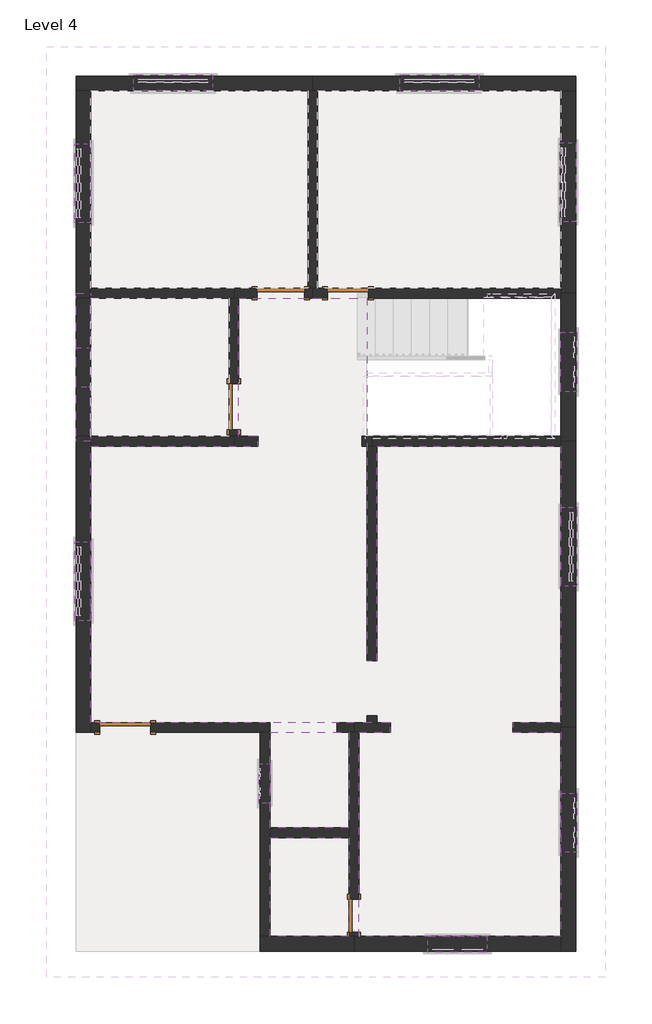
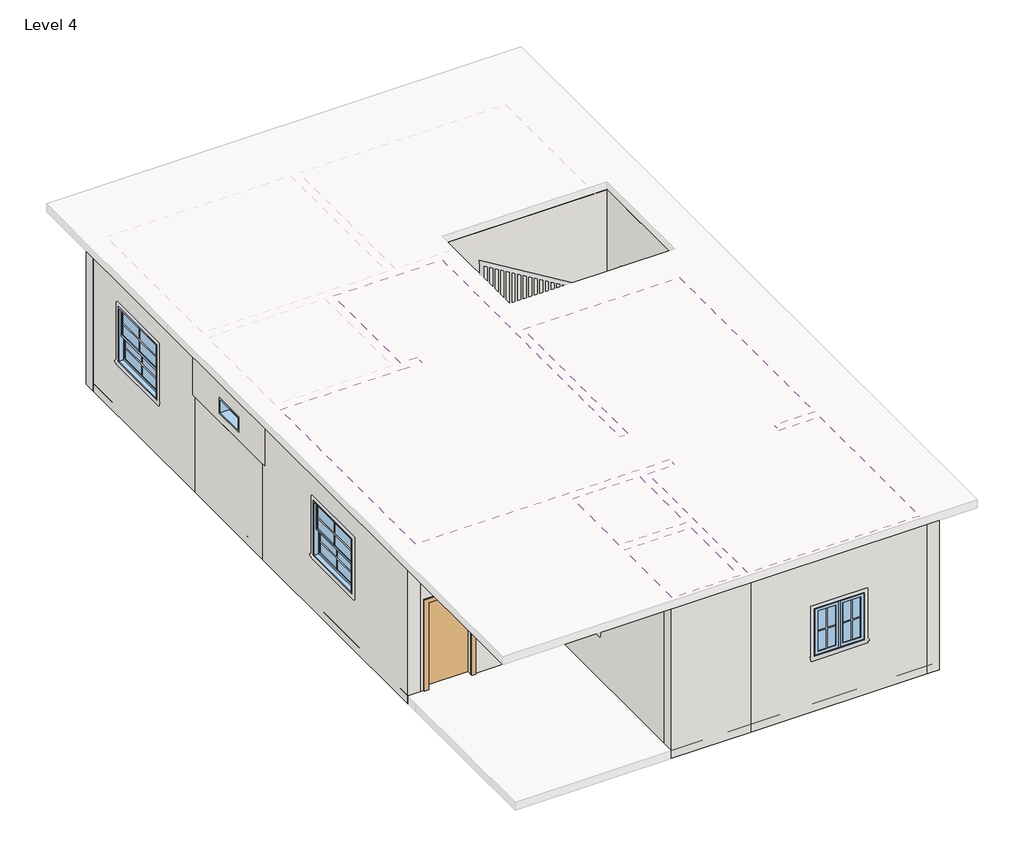
# One storey, part 1 of 2: 26 walls, 11 windows, 5 doors, 3 coverings.
# Revit data of these elements (continued)
# Element 13 (IfcWall, "Generic - 6\"") (continued)
#   built-in parameter 1001111 = 0' - 6"
#   Top Offset = 0' - 0"
#   Base Offset = 0' - 6"
#   Unconnected Height = 10' - 6"
#   wall height = 10' - 6"
#   Phase Created = New Construction
#   Base Constraint = Level 4
#   Materials on its faces: "Default Wall", "DINING ROOM WALL", "BURGUNDY COLOUR"
# Element 15 (IfcWall, "Generic - 6\"")
#   built-in parameter 1001111 = 0' - 6"
#   Top Offset = 0' - 0"
#   Base Offset = 0' - 6"
#   Unconnected Height = 10' - 6"
#   wall height = 10' - 6"
#   Phase Created = New Construction
#   Base Constraint = Level 4
#   Materials on its faces: "Default Wall", "GOLD"
# Element 18 (IfcWall, "Generic - 6\"")
#   built-in parameter 1001111 = 0' - 6"
#   Top Offset = 0' - 0"
#   Base Offset = 0' - 6"
#   Unconnected Height = 10' - 6"
#   wall height = 10' - 6"
#   Phase Created = New Construction
#   Base Constraint = Level 4
#   Materials on its faces: "Default Wall", "DINING ROOM WALL", "LAVENDER WHITE"
# Elements 19, 21 (IfcWall, "Generic - 6\"")
#   built-in parameter 1001111 = 0' - 6"
#   Top Offset = 0' - 0"
#   Base Offset = 0' - 6"
#   Unconnected Height = 10' - 6"
#   wall height = 10' - 6"
#   Phase Created = New Construction
#   Base Constraint = Level 4
#   Materials on its faces: "Default Wall", "DINING ROOM WALL"
# Element 20 (IfcWall, "Generic - 6\"")
#   built-in parameter 1001111 = 0' - 6"
#   Top Offset = 0' - 0"
#   Base Offset = 0' - 6"
#   Unconnected Height = 10' - 6"
#   wall height = 10' - 6"
#   Phase Created = New Construction
#   Base Constraint = Level 4
#   Materials on its faces: "Default Wall", "LIVING ROOM WALL"
# Element 23 (IfcWall, "Generic - 9\"")
#   built-in parameter 1001111 = 0' - 6"
#   Top Offset = 0' - 0"
#   Base Offset = 0' - 6"
#   Unconnected Height = 10' - 6"
#   wall height = 10' - 6"
#   Phase Created = New Construction
#   Base Constraint = Level 4
#   Materials on its faces: "Default Wall", "BURGUNDY COLOUR"
# Elements 24, 26 (IfcWall, "Generic - 9\"")
#   built-in parameter 1001111 = 0' - 6"
#   Top Offset = 0' - 0"
#   Base Offset = 0' - 6"
#   Unconnected Height = 10' - 6"
#   wall height = 10' - 6"
#   Phase Created = New Construction
#   Base Constraint = Level 4
#   Materials on its faces: "Default Wall", "LAVENDER WHITE"
# Element 25 (IfcWall, "Generic - 9\"")
#   built-in parameter 1001111 = 0' - 6"
#   Top Offset = 0' - 0"
#   Base Offset = 0' - 6"
#   Unconnected Height = 10' - 6"
#   wall height = 10' - 6"
#   Phase Created = New Construction
#   Base Constraint = Level 4
#   Materials on its faces: "Default Wall", "GOLD"
# Elements 27, 28, 31, 32 (IfcWall, "Generic - 9\"")
#   built-in parameter 1001111 = 0' - 6"
#   Top Offset = 0' - 0"
#   Base Offset = 0' - 6"
#   Unconnected Height = 10' - 6"
#   wall height = 10' - 6"
#   Phase Created = New Construction
#   Base Constraint = Level 4
#   Materials on its faces: "Default Wall"
# Element 29 (IfcWall, "Generic - 9\"")
#   built-in parameter 1001111 = 0' - 6"
#   Top Offset = 0' - 0"
#   Base Offset = 0' - 6"
#   Unconnected Height = 10' - 6"
#   wall height = 10' - 6"
#   Phase Created = New Construction
#   Base Constraint = Level 4
#   Materials on its faces: "Default Wall", "BURGUNDY COLOUR", "LAVENDER WHITE"
# Element 30 (IfcWall, "Generic - 9\"")
#   built-in parameter 1001111 = 0' - 6"
#   Top Offset = 0' - 0"
#   Base Offset = 0' - 6"
#   Unconnected Height = 10' - 6"
#   wall height = 10' - 6"
#   Phase Created = New Construction
#   Base Constraint = Level 4
#   Materials on its faces: "Default Wall", "DINING ROOM WALL"
# Element 33 (IfcWall, "Generic - 9\"")
#   built-in parameter 1001111 = 6' - 6"
#   Top Offset = 0' - 0"
#   Base Offset = 6' - 6"
#   Unconnected Height = 4' - 6"
#   wall height = 4' - 6"
#   Phase Created = New Construction
#   Base Constraint = Level 4
#   Materials on its faces: "Default Wall", "BATHROOM TILES"
# Element 34 (IfcWall, "Generic - 9\"")
#   built-in parameter 1001111 = 0' - 6"
#   Top Offset = 0' - 0"
#   Base Offset = 0' - 6"
#   Unconnected Height = 6' - 0"
#   wall height = 6' - 0"
#   Phase Created = New Construction
#   Base Constraint = Level 4
#   Materials on its faces: "Default Wall", "BATHROOM TILES"
# Element 35 (IfcWindow, "Fixed : 2'")
#   Mark = "43"
#   Phase Created = New Construction
#   Materials on its faces: "Sash", "Glass"
# Element 36 (IfcWindow, "Window-Casement-Double : 2'")
#   Mark = "42"
#   Window Inset = 0' - 0"
#   Interior Wall Closure = 0' - 2 1/4"
#   Frame Extension = 0' - 0 1/4"
#   Exterior Wall Closure = 0' - 1 1/4"
#   Interior Trim Visibility = yes
#   Exterior Trim Visibility = yes
#   Phase Created = New Construction
#   Materials on its faces: "Wood - Stained", "Glass", "Clad - White"
# Element 37 (IfcWindow, "Window-Casement-Double : 3'")
#   Mark = "40"
#   Window Inset = 0' - 0"
#   Interior Wall Closure = 0' - 2 1/4"
#   Frame Extension = 0' - 0 1/4"
#   Exterior Wall Closure = 0' - 1 1/4"
#   Interior Trim Visibility = yes
#   Exterior Trim Visibility = yes
#   Phase Created = New Construction
#   Materials on its faces: "Wood - Stained", "Glass", "Clad - White"
# Element 38 (IfcWindow, "Window-Casement-Double : 3'")
#   Mark = "41"
#   Window Inset = 0' - 0"
#   Interior Wall Closure = 0' - 2 1/4"
#   Frame Extension = 0' - 0 1/4"
#   Exterior Wall Closure = 0' - 1 1/4"
#   Interior Trim Visibility = yes
#   Exterior Trim Visibility = yes
#   Phase Created = New Construction
#   Materials on its faces: "Wood - Stained", "Glass", "Clad - White"
# Element 39 (IfcWindow, "Window-Casement-Double : 3'")
#   Mark = "44"
#   Window Inset = 0' - 0"
#   Interior Wall Closure = 0' - 2 1/4"
#   Frame Extension = 0' - 0 1/4"
#   Exterior Wall Closure = 0' - 1 1/4"
#   Interior Trim Visibility = yes
#   Exterior Trim Visibility = yes
#   Phase Created = New Construction
#   Materials on its faces: "Wood - Stained", "Glass", "Clad - White"
# Element 40 (IfcWindow, "Window-Double-Hung : 4'")
#   Mark = "36"
#   Window Inset = 0' - 0"
#   Interior Wall Closure = 0' - 1 1/2"
#   Frame Extension = 0' - 1 1/4"
#   Exterior Wall Closure = 0' - 0 1/2"
#   Interior Trim Visibility = yes
#   Indicator Visibility = yes
#   Exterior Trim Visibility = yes
#   Phase Created = New Construction
#   Materials on its faces: "Wood - Stained", "Glass", "Clad - White"
# Element 41 (IfcWindow, "Window-Double-Hung : 4'")
#   Mark = "38"
#   Window Inset = 0' - 0"
#   Interior Wall Closure = 0' - 1 1/2"
#   Frame Extension = 0' - 1 1/4"
#   Exterior Wall Closure = 0' - 0 1/2"
#   Interior Trim Visibility = yes
#   Indicator Visibility = yes
#   Exterior Trim Visibility = yes
#   Phase Created = New Construction
#   Materials on its faces: "Wood - Stained", "Glass", "Clad - White"
# Element 42 (IfcWindow, "Window-Double-Hung : 4'")
#   Mark = "39"
#   Window Inset = 0' - 0"
#   Interior Wall Closure = 0' - 1 1/2"
#   Frame Extension = 0' - 1 1/4"
#   Exterior Wall Closure = 0' - 0 1/2"
#   Interior Trim Visibility = yes
#   Indicator Visibility = yes
#   Exterior Trim Visibility = yes
#   Phase Created = New Construction
#   Materials on its faces: "Wood - Stained", "Glass", "Clad - White"
# Element 43 (IfcWindow, "Window-Double-Hung : 4'")
#   Mark = "34"
#   Window Inset = 0' - 0"
#   Interior Wall Closure = 0' - 1 1/2"
#   Frame Extension = 0' - 1 1/4"
#   Exterior Wall Closure = 0' - 0 1/2"
#   Interior Trim Visibility = yes
#   Indicator Visibility = yes
#   Exterior Trim Visibility = yes
#   Phase Created = New Construction
#   Materials on its faces: "Wood - Stained", "Glass", "Clad - White"
# Element 44 (IfcWindow, "Window-Double-Hung : 4'")
#   Mark = "35"
#   Window Inset = 0' - 0"
#   Interior Wall Closure = 0' - 1 1/2"
#   Frame Extension = 0' - 1 1/4"
#   Exterior Wall Closure = 0' - 0 1/2"
#   Interior Trim Visibility = yes
#   Indicator Visibility = yes
#   Exterior Trim Visibility = yes
#   Phase Created = New Construction
#   Materials on its faces: "Wood - Stained", "Glass", "Clad - White"
# Element 45 (IfcWindow, "Window-Double-Hung : 4'")
#   Mark = "37"
#   Window Inset = 0' - 0"
#   Interior Wall Closure = 0' - 1 1/2"
#   Frame Extension = 0' - 1 1/4"
#   Exterior Wall Closure = 0' - 0 1/2"
#   Interior Trim Visibility = yes
#   Indicator Visibility = yes
#   Exterior Trim Visibility = yes
#   Phase Created = New Construction
#   Materials on its faces: "Wood - Stained", "Glass", "Clad - White"
# Materials
#   "Default": colour RGB 127 127 127, transparency 0, Cost = 0
#   "Acoustic Ceiling Tile 24 x 48": class "Generic", colour RGB 229 229 229, transparency 0, Description = "Acoustic Ceiling Tile 24 x 48", Cost = 0
#   "Door - Panel": class "Wood", colour RGB 210 159 95, transparency 0, Cost = 0
#   "Door - Frame": colour RGB 118 70 51, transparency 0, Cost = 0
#   "Glass": class "Glass", colour RGB 0 128 192, transparency 0.75, Description = "Soda Lime Glass", Cost = 0
#   "Sash": class "Wood", colour RGB 224 178 126, transparency 0, Cost = 0
#   "Wood - Stained": class "Wood", colour RGB 224 178 126, transparency 0, Cost = 0
#   "Clad - White": class "Wood", colour RGB 242 242 238, transparency 0, Cost = 0
#   "Default Wall": colour RGB 128 128 128, transparency 0, Cost = 0
#   "LAVENDER WHITE": class "Generic", colour RGB 120 120 120, transparency 0, Cost = 0
#   "LIVING ROOM WALL": class "Generic", colour RGB 120 120 120, transparency 0, Cost = 0
#   "BURGUNDY COLOUR": class "Generic", colour RGB 120 120 120, transparency 0, Cost = 0
#   "DINING ROOM WALL": class "Generic", colour RGB 120 120 120, transparency 0, Cost = 0
#   "GOLD": class "Generic", colour RGB 120 120 120, transparency 0, Cost = 0
#   "BATHROOM TILES": class "Generic", colour RGB 120 120 120, transparency 0, Cost = 0
